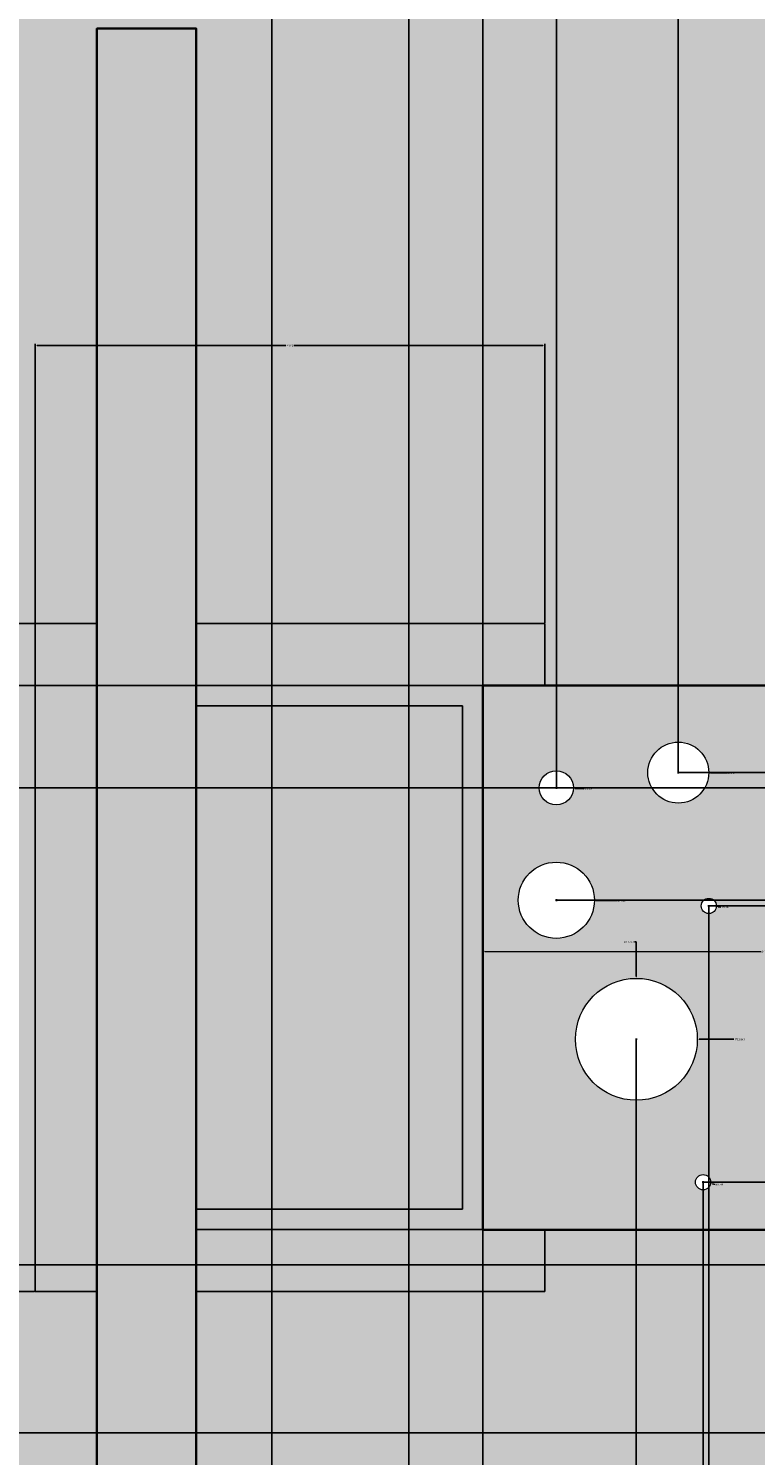
# Model space of a CAD drawing. Units: inches. Extents: x 73 to 607, y 92 to 651.
# Tile 3 of 18: x 298 to 368, y 173 to 311. Entities that reach past the tile are written whole.
import ezdxf

# ---------------------------------------------------------------- set-up
doc = ezdxf.new("R2010")
doc.units = ezdxf.units.IN
doc.header["$MEASUREMENT"] = 0
for name, color, linetype, lineweight in [('A-ANNO-DIMS', 2, 'Continuous', 18), ('A-ELEV', 7, 'Continuous', 35), ('A-ELEV-PANL', 7, 'Continuous', 18), ('A-ELEV-PATT-BKGD', 252, 'Continuous', 13), ('A-ELEV-PATT-FRAM', 38, 'Continuous', 13), ('A-ELEV-PATT-SHAD', 8, 'Continuous', 13), ('A-ELEV-PATT-WALL', 254, 'Continuous', 13), ('A-ELEV-PATT-WOOD', 32, 'Continuous', 13), ('A-GLAZ', 4, 'Continuous', 25), ('A-GLAZ-PATT', 7, 'Continuous', 13)]:
    doc.layers.add(name, color=color, linetype=linetype, lineweight=lineweight)
doc.styles.get("Standard").update_dxf_attribs({"font": 'arial.ttf'})
doc.dimstyles.get("Standard").update_dxf_attribs({"dimtxt": 0.18, "dimasz": 0.18, "dimexe": 0.18, "dimexo": 0.0625, "dimgap": 0.09, "dimtad": 0, "dimtih": 1, "dimtoh": 1, "dimdec": 4, "dimzin": 0, "dimdsep": 46, "dimtxsty": 'Standard', "dimcen": 0.09, "dimadec": 0, "dimazin": 0, "dimtfac": 1, "dimtdec": 4, "dimtofl": 0, "dimtmove": 0, "dimatfit": 3, "dimfxl": 1, "dimtolj": 1, "dimtzin": 0, "dimarcsym": 0})

# ---------------------------------------------------------------- blocks, each defined once
blk = doc.blocks.new('*D33')
at = {"layer": 'A-ANNO-DIMS', "color": 0, "lineweight": -2, "transparency": 16777216}
for p, q in [((298.36, 253.47), (298.36, 280.59)), ((298.54, 280.41), (322.73, 280.41)), ((347.69, 280.41), (323.49, 280.41)), ((347.87, 253.47), (347.87, 280.59))]:
    blk.add_line(p, q, dxfattribs=at)
at = {"layer": 'A-ANNO-DIMS', "color": 0, "transparency": 16777216}
for points in [[(298.54, 280.44), (298.54, 280.38), (298.36, 280.41)], [(347.69, 280.44), (347.69, 280.38), (347.87, 280.41)]]:
    blk.add_solid(points, dxfattribs=at)
at = {"layer": 'Defpoints', "color": 0, "transparency": 16777216}
for p in [(347.87, 280.41), (298.36, 253.41), (347.87, 253.41)]:
    blk.add_point(p, dxfattribs=at)
at = {"layer": 'A-ANNO-DIMS', "color": 0, "transparency": 16777216, "insert": (323.11, 280.41), "char_height": 0.18, "attachment_point": 5}
blk.add_mtext('\\A1;49.51', dxfattribs=at)
blk = doc.blocks.new('*D34')
at = {"layer": 'A-ANNO-DIMS', "color": 0, "lineweight": -2, "transparency": 16777216}
for p, q in [((298.29, 253.41), (271.18, 253.41)), ((271.36, 253.23), (271.36, 221.16)), ((271.36, 188.73), (271.36, 220.79)), ((298.29, 188.55), (271.18, 188.55))]:
    blk.add_line(p, q, dxfattribs=at)
at = {"layer": 'A-ANNO-DIMS', "color": 0, "transparency": 16777216}
for points in [[(271.33, 253.23), (271.39, 253.23), (271.36, 253.41)], [(271.33, 188.73), (271.39, 188.73), (271.36, 188.55)]]:
    blk.add_solid(points, dxfattribs=at)
at = {"layer": 'Defpoints', "color": 0, "transparency": 16777216}
for p in [(271.36, 253.41), (298.36, 253.41), (298.36, 188.55)]:
    blk.add_point(p, dxfattribs=at)
at = {"layer": 'A-ANNO-DIMS', "color": 0, "transparency": 16777216, "insert": (271.36, 220.98), "char_height": 0.18, "attachment_point": 5}
blk.add_mtext('\\A1;64.86', dxfattribs=at)
blk = doc.blocks.new('*D35')
at = {"layer": 'A-ANNO-DIMS', "color": 0, "lineweight": -2, "transparency": 16777216}
for p, q in [((341.87, 194.61), (341.87, 221.73)), ((342.05, 221.55), (368.89, 221.54)), ((396.52, 221.54), (369.68, 221.54)), ((396.69, 194.6), (396.7, 221.72))]:
    blk.add_line(p, q, dxfattribs=at)
at = {"layer": 'A-ANNO-DIMS', "color": 0, "transparency": 16777216}
for points in [[(342.05, 221.58), (342.05, 221.52), (341.87, 221.55)], [(396.52, 221.57), (396.52, 221.51), (396.7, 221.54)]]:
    blk.add_solid(points, dxfattribs=at)
at = {"layer": 'Defpoints', "color": 0, "transparency": 16777216}
for p in [(396.7, 221.54), (341.87, 194.55), (396.69, 194.54)]:
    blk.add_point(p, dxfattribs=at)
at = {"layer": 'A-ANNO-DIMS', "color": 0, "transparency": 16777216, "insert": (369.28, 221.54), "char_height": 0.18, "attachment_point": 5}
blk.add_mtext('\\A1;54.82', dxfattribs=at)
blk = doc.blocks.new('*D66')
at = {"layer": 'A-ANNO-DIMS', "color": 0, "lineweight": -2, "transparency": 16777216}
for p, q in [((356.68, 213.03), (356.86, 213.03)), ((356.77, 212.94), (356.77, 213.12)), ((366.25, 213.03), (362.88, 213.03))]:
    blk.add_line(p, q, dxfattribs=at)
at = {"layer": 'A-ANNO-DIMS', "color": 0, "transparency": 16777216}
blk.add_solid([(362.88, 213.06), (362.88, 213), (362.7, 213.03)], dxfattribs=at)
at = {"layer": 'Defpoints', "color": 0, "transparency": 16777216}
for p in [(350.85, 213.03), (362.7, 213.03)]:
    blk.add_point(p, dxfattribs=at)
at = {"layer": 'A-ANNO-DIMS', "color": 0, "transparency": 16777216, "insert": (366.81, 213.03), "char_height": 0.18, "attachment_point": 5}
blk.add_mtext('\\A1;∅11.843', dxfattribs=at)
blk = doc.blocks.new('*D77')
at = {"layer": 'A-ANNO-DIMS', "color": 0, "lineweight": -2, "transparency": 16777216}
for p, q in [((321.37, 356.99), (321.37, 116.02)), ((334.67, 320.14), (334.67, 116.02)), ((321.55, 116.2), (327.63, 116.2)), ((334.49, 116.2), (328.4, 116.2))]:
    blk.add_line(p, q, dxfattribs=at)
at = {"layer": 'A-ANNO-DIMS', "color": 0, "transparency": 16777216}
for points in [[(321.55, 116.23), (321.55, 116.17), (321.37, 116.2)], [(334.49, 116.23), (334.49, 116.17), (334.67, 116.2)]]:
    blk.add_solid(points, dxfattribs=at)
at = {"layer": 'Defpoints', "color": 0, "transparency": 16777216}
for p in [(321.37, 357.06), (334.67, 320.2), (321.37, 116.2)]:
    blk.add_point(p, dxfattribs=at)
at = {"layer": 'A-ANNO-DIMS', "color": 0, "transparency": 16777216, "insert": (328.02, 116.2), "char_height": 0.18, "attachment_point": 5}
blk.add_mtext('\\A1;13.30', dxfattribs=at)
blk = doc.blocks.new('*D81')
at = {"layer": 'A-ANNO-DIMS', "color": 0, "lineweight": -2, "transparency": 16777216}
for p, q in [((341.87, 247.47), (341.87, 650.98)), ((342.05, 650.8), (345.04, 650.8)), ((348.82, 650.8), (345.83, 650.8)), ((349, 237.52), (349, 650.98))]:
    blk.add_line(p, q, dxfattribs=at)
at = {"layer": 'A-ANNO-DIMS', "color": 0, "transparency": 16777216}
for points in [[(342.05, 650.83), (342.05, 650.77), (341.87, 650.8)], [(348.82, 650.83), (348.82, 650.77), (349, 650.8)]]:
    blk.add_solid(points, dxfattribs=at)
at = {"layer": 'Defpoints', "color": 0, "transparency": 16777216}
for p in [(349, 650.8), (341.87, 247.41), (349, 237.45)]:
    blk.add_point(p, dxfattribs=at)
at = {"layer": 'A-ANNO-DIMS', "color": 0, "transparency": 16777216, "insert": (345.43, 650.8), "char_height": 0.18, "attachment_point": 5}
blk.add_mtext('\\A1;7.128', dxfattribs=at)
blk = doc.blocks.new('*D82')
at = {"layer": 'A-ANNO-DIMS', "color": 0, "lineweight": -2, "transparency": 16777216}
for p, q in [((349, 237.52), (349, 650.98)), ((349.18, 650.8), (354.47, 650.8)), ((360.67, 650.8), (355.38, 650.8)), ((360.85, 239), (360.85, 650.98))]:
    blk.add_line(p, q, dxfattribs=at)
at = {"layer": 'A-ANNO-DIMS', "color": 0, "transparency": 16777216}
for points in [[(349.18, 650.83), (349.18, 650.77), (349, 650.8)], [(360.67, 650.83), (360.67, 650.77), (360.85, 650.8)]]:
    blk.add_solid(points, dxfattribs=at)
at = {"layer": 'Defpoints', "color": 0, "transparency": 16777216}
for p in [(360.85, 650.8), (360.85, 238.93), (349, 237.45)]:
    blk.add_point(p, dxfattribs=at)
at = {"layer": 'A-ANNO-DIMS', "color": 0, "transparency": 16777216, "insert": (354.92, 650.8), "char_height": 0.18, "attachment_point": 5}
blk.add_mtext('\\A1;11.852', dxfattribs=at)
blk = doc.blocks.new('*D83')
at = {"layer": 'A-ANNO-DIMS', "color": 0, "lineweight": -2, "transparency": 16777216}
for p, q in [((360.85, 239), (360.85, 650.98)), ((361.03, 650.8), (366.6, 650.8)), ((373.08, 650.8), (367.51, 650.8)), ((373.26, 231.41), (373.26, 650.98))]:
    blk.add_line(p, q, dxfattribs=at)
at = {"layer": 'A-ANNO-DIMS', "color": 0, "transparency": 16777216}
for points in [[(361.03, 650.83), (361.03, 650.77), (360.85, 650.8)], [(373.08, 650.83), (373.08, 650.77), (373.26, 650.8)]]:
    blk.add_solid(points, dxfattribs=at)
at = {"layer": 'Defpoints', "color": 0, "transparency": 16777216}
for p in [(373.26, 650.8), (360.85, 238.93), (373.26, 231.35)]:
    blk.add_point(p, dxfattribs=at)
at = {"layer": 'A-ANNO-DIMS', "color": 0, "transparency": 16777216, "insert": (367.05, 650.8), "char_height": 0.18, "attachment_point": 5}
blk.add_mtext('\\A1;12.408', dxfattribs=at)
blk = doc.blocks.new('*D86')
at = {"layer": 'A-ANNO-DIMS', "color": 0, "lineweight": -2, "transparency": 16777216}
for p, q in [((356.77, 212.97), (356.77, 116.02)), ((341.87, 194.47), (341.87, 116.02)), ((342.05, 116.2), (348.87, 116.2)), ((356.59, 116.2), (349.78, 116.2))]:
    blk.add_line(p, q, dxfattribs=at)
at = {"layer": 'A-ANNO-DIMS', "color": 0, "transparency": 16777216}
for points in [[(342.05, 116.23), (342.05, 116.17), (341.87, 116.2)], [(356.59, 116.23), (356.59, 116.17), (356.77, 116.2)]]:
    blk.add_solid(points, dxfattribs=at)
at = {"layer": 'Defpoints', "color": 0, "transparency": 16777216}
for p in [(356.77, 213.03), (341.87, 194.54), (356.77, 116.2)]:
    blk.add_point(p, dxfattribs=at)
at = {"layer": 'A-ANNO-DIMS', "color": 0, "transparency": 16777216, "insert": (349.32, 116.2), "char_height": 0.18, "attachment_point": 5}
blk.add_mtext('\\A1;14.906', dxfattribs=at)
blk = doc.blocks.new('*D87')
at = {"layer": 'A-ANNO-DIMS', "color": 0, "lineweight": -2, "transparency": 16777216}
for p, q in [((356.77, 212.97), (356.77, 116.02)), ((363.26, 199.09), (363.26, 116.02)), ((356.95, 116.2), (359.62, 116.2)), ((363.08, 116.2), (360.41, 116.2))]:
    blk.add_line(p, q, dxfattribs=at)
at = {"layer": 'A-ANNO-DIMS', "color": 0, "transparency": 16777216}
for points in [[(356.95, 116.23), (356.95, 116.17), (356.77, 116.2)], [(363.08, 116.23), (363.08, 116.17), (363.26, 116.2)]]:
    blk.add_solid(points, dxfattribs=at)
at = {"layer": 'Defpoints', "color": 0, "transparency": 16777216}
for p in [(356.77, 213.03), (363.26, 199.15), (363.26, 116.2)]:
    blk.add_point(p, dxfattribs=at)
at = {"layer": 'A-ANNO-DIMS', "color": 0, "transparency": 16777216, "insert": (360.02, 116.2), "char_height": 0.18, "attachment_point": 5}
blk.add_mtext('\\A1;6.482', dxfattribs=at)
blk = doc.blocks.new('*D88')
at = {"layer": 'A-ANNO-DIMS', "color": 0, "lineweight": -2, "transparency": 16777216}
for p, q in [((376.96, 209.08), (376.96, 116.02)), ((363.26, 199.09), (363.26, 116.02)), ((363.44, 116.2), (369.65, 116.2)), ((376.78, 116.2), (370.56, 116.2))]:
    blk.add_line(p, q, dxfattribs=at)
at = {"layer": 'A-ANNO-DIMS', "color": 0, "transparency": 16777216}
for points in [[(363.44, 116.23), (363.44, 116.17), (363.26, 116.2)], [(376.78, 116.23), (376.78, 116.17), (376.96, 116.2)]]:
    blk.add_solid(points, dxfattribs=at)
at = {"layer": 'Defpoints', "color": 0, "transparency": 16777216}
for p in [(376.96, 209.14), (363.26, 199.15), (376.96, 116.2)]:
    blk.add_point(p, dxfattribs=at)
at = {"layer": 'A-ANNO-DIMS', "color": 0, "transparency": 16777216, "insert": (370.11, 116.2), "char_height": 0.18, "attachment_point": 5}
blk.add_mtext('\\A1;13.704', dxfattribs=at)
blk = doc.blocks.new('*D91')
at = {"layer": 'A-ANNO-DIMS', "color": 0, "lineweight": -2, "transparency": 16777216}
for p, q in [((363.81, 225.92), (363.81, 116.02)), ((356.77, 212.97), (356.77, 116.02)), ((356.95, 116.2), (359.9, 116.2)), ((363.63, 116.2), (360.69, 116.2))]:
    blk.add_line(p, q, dxfattribs=at)
at = {"layer": 'A-ANNO-DIMS', "color": 0, "transparency": 16777216}
for points in [[(356.95, 116.23), (356.95, 116.17), (356.77, 116.2)], [(363.63, 116.23), (363.63, 116.17), (363.81, 116.2)]]:
    blk.add_solid(points, dxfattribs=at)
at = {"layer": 'Defpoints', "color": 0, "transparency": 16777216}
for p in [(363.81, 225.98), (356.77, 213.03), (363.81, 116.2)]:
    blk.add_point(p, dxfattribs=at)
at = {"layer": 'A-ANNO-DIMS', "color": 0, "transparency": 16777216, "insert": (360.29, 116.2), "char_height": 0.18, "attachment_point": 5}
blk.add_mtext('\\A1;7.037', dxfattribs=at)
blk = doc.blocks.new('*D92')
at = {"layer": 'A-ANNO-DIMS', "color": 0, "lineweight": -2, "transparency": 16777216}
for p, q in [((341.81, 247.41), (72.92, 247.41)), ((73.1, 247.23), (73.1, 242.61)), ((73.1, 237.63), (73.1, 242.25)), ((348.93, 237.45), (72.92, 237.45))]:
    blk.add_line(p, q, dxfattribs=at)
at = {"layer": 'A-ANNO-DIMS', "color": 0, "transparency": 16777216}
for points in [[(73.07, 247.23), (73.13, 247.23), (73.1, 247.41)], [(73.07, 237.63), (73.13, 237.63), (73.1, 237.45)]]:
    blk.add_solid(points, dxfattribs=at)
at = {"layer": 'Defpoints', "color": 0, "transparency": 16777216}
for p in [(341.87, 247.41), (73.1, 237.45), (349, 237.45)]:
    blk.add_point(p, dxfattribs=at)
at = {"layer": 'A-ANNO-DIMS', "color": 0, "transparency": 16777216, "insert": (73.1, 242.43), "char_height": 0.18, "attachment_point": 5}
blk.add_mtext('\\A1;9.95', dxfattribs=at)
blk = doc.blocks.new('*D93')
at = {"layer": 'A-ANNO-DIMS', "color": 0, "lineweight": -2, "transparency": 16777216}
for p, q in [((349.06, 237.45), (607.28, 237.45)), ((607.1, 237.27), (607.1, 232.18)), ((607.1, 226.72), (607.1, 231.81)), ((349.06, 226.54), (607.28, 226.54))]:
    blk.add_line(p, q, dxfattribs=at)
at = {"layer": 'A-ANNO-DIMS', "color": 0, "transparency": 16777216}
for points in [[(607.07, 237.27), (607.13, 237.27), (607.1, 237.45)], [(607.07, 226.72), (607.13, 226.72), (607.1, 226.54)]]:
    blk.add_solid(points, dxfattribs=at)
at = {"layer": 'Defpoints', "color": 0, "transparency": 16777216}
for p in [(349, 237.45), (349, 226.54), (607.1, 226.54)]:
    blk.add_point(p, dxfattribs=at)
at = {"layer": 'A-ANNO-DIMS', "color": 0, "transparency": 16777216, "insert": (607.1, 232), "char_height": 0.18, "attachment_point": 5}
blk.add_mtext('\\A1;10.917', dxfattribs=at)
blk = doc.blocks.new('*D94')
at = {"layer": 'A-ANNO-DIMS', "color": 0, "lineweight": -2, "transparency": 16777216}
for p, q in [((377.02, 209.14), (607.28, 209.14)), ((607.1, 208.96), (607.1, 204.33)), ((607.1, 199.33), (607.1, 203.97)), ((363.32, 199.15), (607.28, 199.15))]:
    blk.add_line(p, q, dxfattribs=at)
at = {"layer": 'A-ANNO-DIMS', "color": 0, "transparency": 16777216}
for points in [[(607.07, 208.96), (607.13, 208.96), (607.1, 209.14)], [(607.07, 199.33), (607.13, 199.33), (607.1, 199.15)]]:
    blk.add_solid(points, dxfattribs=at)
at = {"layer": 'Defpoints', "color": 0, "transparency": 16777216}
for p in [(376.96, 209.14), (363.26, 199.15), (607.1, 199.15)]:
    blk.add_point(p, dxfattribs=at)
at = {"layer": 'A-ANNO-DIMS', "color": 0, "transparency": 16777216, "insert": (607.1, 204.15), "char_height": 0.18, "attachment_point": 5}
blk.add_mtext('\\A1;9.992', dxfattribs=at)
blk = doc.blocks.new('*D95')
at = {"layer": 'A-ANNO-DIMS', "color": 0, "lineweight": -2, "transparency": 16777216}
for p, q in [((363.87, 225.98), (607.28, 225.98)), ((607.1, 225.8), (607.1, 212.75)), ((607.1, 199.33), (607.1, 212.38)), ((363.32, 199.15), (607.28, 199.15))]:
    blk.add_line(p, q, dxfattribs=at)
at = {"layer": 'A-ANNO-DIMS', "color": 0, "transparency": 16777216}
for points in [[(607.07, 225.8), (607.13, 225.8), (607.1, 225.98)], [(607.07, 199.33), (607.13, 199.33), (607.1, 199.15)]]:
    blk.add_solid(points, dxfattribs=at)
at = {"layer": 'Defpoints', "color": 0, "transparency": 16777216}
for p in [(363.81, 225.98), (607.1, 225.98), (363.26, 199.15)]:
    blk.add_point(p, dxfattribs=at)
at = {"layer": 'A-ANNO-DIMS', "color": 0, "transparency": 16777216, "insert": (607.1, 212.57), "char_height": 0.18, "attachment_point": 5}
blk.add_mtext('\\A1;26.83', dxfattribs=at)
blk = doc.blocks.new('*D96')
at = {"layer": 'A-ANNO-DIMS', "color": 0, "lineweight": -2, "transparency": 16777216}
for p, q in [((360.91, 238.93), (607.28, 238.93)), ((607.1, 238.75), (607.1, 232.64)), ((607.1, 226.16), (607.1, 232.28)), ((363.87, 225.98), (607.28, 225.98))]:
    blk.add_line(p, q, dxfattribs=at)
at = {"layer": 'A-ANNO-DIMS', "color": 0, "transparency": 16777216}
for points in [[(607.07, 238.75), (607.13, 238.75), (607.1, 238.93)], [(607.07, 226.16), (607.13, 226.16), (607.1, 225.98)]]:
    blk.add_solid(points, dxfattribs=at)
at = {"layer": 'Defpoints', "color": 0, "transparency": 16777216}
for p in [(360.85, 238.93), (607.1, 238.93), (363.81, 225.98)]:
    blk.add_point(p, dxfattribs=at)
at = {"layer": 'A-ANNO-DIMS', "color": 0, "transparency": 16777216, "insert": (607.1, 232.46), "char_height": 0.18, "attachment_point": 5}
blk.add_mtext('\\A1;12.953', dxfattribs=at)
blk = doc.blocks.new('*D119')
at = {"layer": 'A-ANNO-DIMS', "color": 0, "lineweight": -2, "transparency": 16777216}
for p, q in [((469.82, 191.14), (72.92, 191.14)), ((73.1, 190.96), (73.1, 183.15)), ((73.1, 174.98), (73.1, 182.79)), ((454.64, 174.8), (72.92, 174.8))]:
    blk.add_line(p, q, dxfattribs=at)
at = {"layer": 'A-ANNO-DIMS', "color": 0, "transparency": 16777216}
for points in [[(73.07, 190.96), (73.13, 190.96), (73.1, 191.14)], [(73.07, 174.98), (73.13, 174.98), (73.1, 174.8)]]:
    blk.add_solid(points, dxfattribs=at)
at = {"layer": 'Defpoints', "color": 0, "transparency": 16777216}
for p in [(73.1, 191.14), (469.88, 191.14), (454.7, 174.8)]:
    blk.add_point(p, dxfattribs=at)
at = {"layer": 'A-ANNO-DIMS', "color": 0, "transparency": 16777216, "insert": (73.1, 182.97), "char_height": 0.18, "attachment_point": 5}
blk.add_mtext('\\A1;16.34', dxfattribs=at)
blk = doc.blocks.new('*D142')
at = {"layer": 'A-ANNO-DIMS', "color": 0, "lineweight": -2, "transparency": 16777216}
for p, q in [((348.91, 237.45), (349.09, 237.45)), ((349, 237.36), (349, 237.54)), ((351.66, 237.37), (350.84, 237.39))]:
    blk.add_line(p, q, dxfattribs=at)
at = {"layer": 'A-ANNO-DIMS', "color": 0, "transparency": 16777216}
blk.add_solid([(350.84, 237.42), (350.84, 237.36), (350.66, 237.4)], dxfattribs=at)
at = {"layer": 'Defpoints', "color": 0, "transparency": 16777216}
for p in [(347.33, 237.51), (350.66, 237.4)]:
    blk.add_point(p, dxfattribs=at)
at = {"layer": 'A-ANNO-DIMS', "color": 0, "transparency": 16777216, "insert": (352.08, 237.37), "char_height": 0.18, "attachment_point": 5}
blk.add_mtext('\\A1;∅3.33', dxfattribs=at)
blk = doc.blocks.new('*D143')
at = {"layer": 'A-ANNO-DIMS', "color": 0, "lineweight": -2, "transparency": 16777216}
for p, q in [((360.76, 238.93), (360.94, 238.93)), ((360.85, 238.84), (360.85, 239.02)), ((365.59, 238.88), (363.99, 238.9))]:
    blk.add_line(p, q, dxfattribs=at)
at = {"layer": 'A-ANNO-DIMS', "color": 0, "transparency": 16777216}
blk.add_solid([(363.99, 238.93), (363.99, 238.87), (363.81, 238.9)], dxfattribs=at)
at = {"layer": 'Defpoints', "color": 0, "transparency": 16777216}
for p in [(357.89, 238.97), (363.81, 238.9)]:
    blk.add_point(p, dxfattribs=at)
at = {"layer": 'A-ANNO-DIMS', "color": 0, "transparency": 16777216, "insert": (366.06, 238.88), "char_height": 0.18, "attachment_point": 5}
blk.add_mtext('\\A1;∅5.921', dxfattribs=at)
blk = doc.blocks.new('*D147')
at = {"layer": 'A-ANNO-DIMS', "color": 0, "lineweight": -2, "transparency": 16777216}
for p, q in [((348.91, 226.54), (349.09, 226.54)), ((349, 226.45), (349, 226.63)), ((354.92, 226.48), (352.88, 226.5))]:
    blk.add_line(p, q, dxfattribs=at)
at = {"layer": 'A-ANNO-DIMS', "color": 0, "transparency": 16777216}
blk.add_solid([(352.88, 226.53), (352.88, 226.47), (352.7, 226.5)], dxfattribs=at)
at = {"layer": 'Defpoints', "color": 0, "transparency": 16777216}
for p in [(345.3, 226.57), (352.7, 226.5)]:
    blk.add_point(p, dxfattribs=at)
at = {"layer": 'A-ANNO-DIMS', "color": 0, "transparency": 16777216, "insert": (355.41, 226.48), "char_height": 0.18, "attachment_point": 5}
blk.add_mtext('\\A1;∅7.402', dxfattribs=at)
blk = doc.blocks.new('*D148')
at = {"layer": 'A-ANNO-DIMS', "color": 0, "lineweight": -2, "transparency": 16777216}
for p, q in [((363.72, 225.98), (363.9, 225.98)), ((363.81, 225.89), (363.81, 226.07)), ((364.99, 225.86), (364.73, 225.89))]:
    blk.add_line(p, q, dxfattribs=at)
at = {"layer": 'A-ANNO-DIMS', "color": 0, "transparency": 16777216}
blk.add_solid([(364.73, 225.92), (364.72, 225.86), (364.55, 225.91)], dxfattribs=at)
at = {"layer": 'Defpoints', "color": 0, "transparency": 16777216}
for p in [(363.08, 226.06), (364.55, 225.91)]:
    blk.add_point(p, dxfattribs=at)
at = {"layer": 'A-ANNO-DIMS', "color": 0, "transparency": 16777216, "insert": (365.41, 225.86), "char_height": 0.18, "attachment_point": 5}
blk.add_mtext('\\A1;∅1.48', dxfattribs=at)
blk = doc.blocks.new('*D150')
at = {"layer": 'A-ANNO-DIMS', "color": 0, "lineweight": -2, "transparency": 16777216}
for p, q in [((356.59, 222.5), (356.77, 222.5)), ((356.77, 222.5), (356.77, 219.13)), ((356.68, 213.03), (356.86, 213.03)), ((356.77, 212.94), (356.77, 213.12))]:
    blk.add_line(p, q, dxfattribs=at)
at = {"layer": 'A-ANNO-DIMS', "color": 0, "transparency": 16777216}
blk.add_solid([(356.8, 219.13), (356.74, 219.13), (356.77, 218.95)], dxfattribs=at)
at = {"layer": 'Defpoints', "color": 0, "transparency": 16777216}
for p in [(356.77, 218.95), (356.78, 207.11)]:
    blk.add_point(p, dxfattribs=at)
at = {"layer": 'A-ANNO-DIMS', "color": 0, "transparency": 16777216, "insert": (356.03, 222.5), "char_height": 0.18, "attachment_point": 5}
blk.add_mtext('\\A1;∅11.843', dxfattribs=at)
blk = doc.blocks.new('*D152')
at = {"layer": 'A-ANNO-DIMS', "color": 0, "lineweight": -2, "transparency": 16777216}
for p, q in [((363.17, 199.15), (363.35, 199.15)), ((363.26, 199.06), (363.26, 199.24)), ((364.42, 198.93), (364.16, 198.98))]:
    blk.add_line(p, q, dxfattribs=at)
at = {"layer": 'A-ANNO-DIMS', "color": 0, "transparency": 16777216}
blk.add_solid([(364.17, 199.01), (364.16, 198.95), (363.98, 199.01)], dxfattribs=at)
at = {"layer": 'Defpoints', "color": 0, "transparency": 16777216}
for p in [(362.53, 199.29), (363.98, 199.01)]:
    blk.add_point(p, dxfattribs=at)
at = {"layer": 'A-ANNO-DIMS', "color": 0, "transparency": 16777216, "insert": (364.84, 198.93), "char_height": 0.18, "attachment_point": 5}
blk.add_mtext('\\A1;∅1.48', dxfattribs=at)

msp = doc.modelspace()

# ---------------------------------------------------------------- hatches: boundary and pattern name
at = {"layer": 'A-ELEV-PATT-BKGD'}
h = msp.add_hatch(color=256, dxfattribs=at)
h.dxf.hatch_style = 1
h.paths.add_polyline_path([(321.3008, 479.2042), (312.3008, 479.2042), (312.3008, 478.7576), (312.3008, 412.636), (321.3008, 412.636)])
h.paths.add_polyline_path([(312.3008, 504.7576), (256.4726, 504.7576), (256.4726, 503.4576), (312.3008, 503.4576)], flags=17)
h.paths.add_polyline_path([(321.3008, 543.1576), (321.3008, 552.1576), (320.3257, 552.1576), (312.3008, 552.1576), (256.4726, 552.1576), (256.4726, 543.1576), (312.3008, 543.1576), (312.3008, 479.2042), (321.3008, 479.2042)])
h.paths.add_polyline_path([(451.5214, 412.636), (256.4726, 412.636), (256.4726, 403.636), (442.5214, 403.636), (442.5214, 320.2042), (206.1343, 320.2042), (206.1343, 320.9135), (206.1343, 403.636), (256.4726, 403.636), (256.4726, 412.636), (201.6343, 412.636), (201.6343, 320.9135), (201.6343, 320.2042), (201.6343, 311.2042), (256.4726, 311.2042), (451.5214, 311.2042)])
h.paths.add_polyline_path([(431.07, 258.6914), (369.5339, 258.6914), (369.5339, 247.4054), (396.692, 247.4054), (425.07, 247.4054), (425.07, 194.7312), (396.692, 194.6197), (396.692, 194.5366), (369.5339, 194.5366), (369.5339, 185.6619), (431.07, 185.6619)])
h.paths.add_polyline_path([(580.0983, 262.3024), (451.5214, 262.3024), (451.5214, 143.2042), (580.0983, 143.2042)])
h.paths.add_polyline_path([(454.7049, 174.802), (454.7049, 256.6321), (577.9249, 256.6321), (577.9249, 174.802)], flags=16)
h.paths.add_polyline_path([(465.9716, 191.1416, -1), (473.7874, 191.1416, -1)], flags=0)
h.paths.add_polyline_path([(490.5373, 181.6586, -1), (494.9999, 181.6586, -1)], flags=0)
h.paths.add_polyline_path([(476.2996, 209.8287, -1), (500.5844, 209.8287, -1)], flags=0)
h.paths.add_polyline_path([(505.3326, 194.7675, -1), (512.5843, 194.7675, -1)], flags=0)
h.paths.add_polyline_path([(520.9613, 186.679, -1), (526.544, 186.679, -1)], flags=0)
h.paths.add_polyline_path([(466.8103, 225.7267, -1), (470.1573, 225.7267, -1)], flags=0)
h.paths.add_polyline_path([(527.1059, 203.6926, -1), (536.0311, 203.6926, -1)], flags=0)
h.paths.add_polyline_path([(504.775, 232.6995, -1), (513.7002, 232.6995, -1)], flags=0)
h.paths.add_polyline_path([(546.9241, 183.611, -1), (554.7336, 183.611, -1)], flags=0)
h.paths.add_polyline_path([(459.5544, 243.856, -1), (466.8061, 243.856, -1)], flags=0)
h.paths.add_polyline_path([(476.3045, 246.924, -1), (488.5767, 246.924, -1)], flags=0)
h.paths.add_polyline_path([(529.9044, 226.8424, -1), (556.68, 226.8424, -1)], flags=0)
h.paths.add_polyline_path([(554.1814, 203.9716, -1), (561.4331, 203.9716, -1)], flags=0)
h.paths.add_polyline_path([(567.8561, 193.3729, -1), (570.6475, 193.3729, -1)], flags=0)
h.paths.add_polyline_path([(522.3584, 250.271, -1), (525.7053, 250.271, -1)], flags=0)
h.paths.add_polyline_path([(561.9965, 245.2506, -1), (567.5748, 245.2506, -1)], flags=0)
h.paths.add_polyline_path([(347.8686, 194.5366), (341.8686, 194.5366), (341.8686, 194.5452), (314.0144, 194.5452), (314.0144, 188.5452), (347.8686, 188.5452)])
h.paths.add_polyline_path([(347.8686, 253.4054), (314.0144, 253.4054), (314.0144, 247.4054), (341.8686, 247.4054), (347.8686, 247.4054)])
h.paths.add_polyline_path([(304.3559, 253.4054), (298.3559, 253.4054), (298.3559, 188.5452), (304.3559, 188.5452)])
h.paths.add_polyline_path([(450.6603, 552.1576), (369.9727, 552.1576), (369.9727, 479.2042), (374.4727, 479.2042), (374.4727, 547.6576), (446.1603, 547.6576), (446.1603, 479.2042), (450.6603, 479.2042)])
h.paths.add_polyline_path([(374.4727, 479.2042), (369.9727, 479.2042), (369.9727, 465.0632), (374.4727, 465.0632)])
h.paths.add_polyline_path([(450.6603, 479.2042), (446.1603, 479.2042), (446.1603, 465.0632), (450.6603, 465.0632)])
h.paths.add_polyline_path([(256.4726, 281.6039), (109.0983, 281.6039), (100.0983, 281.6039), (100.0983, 167.2042), (100.0983, 143.2042), (109.0983, 143.2042), (109.0983, 167.2042), (109.0983, 272.6039), (256.4726, 272.6039)])
at = {"layer": 'A-ELEV-PATT-FRAM'}
h = msp.add_hatch(color=256, dxfattribs=at)
h.dxf.hatch_style = 1
h.paths.add_polyline_path([(433.025, 403.636), (409.515, 403.636), (409.515, 342.1009), (411.515, 342.1009), (411.515, 401.636), (431.025, 401.636), (431.025, 342.1009), (433.025, 342.1009)])
h.paths.add_polyline_path([(433.025, 341.1009), (431.025, 341.1009), (431.025, 340.0025), (411.515, 340.0025), (411.515, 341.1009), (409.515, 341.1009), (409.515, 338.0025), (433.025, 338.0025)])
h.paths.add_polyline_path([(425.07, 247.4054), (396.692, 247.4054), (396.692, 194.6197), (425.07, 194.7312)])
h.paths.add_polyline_path([(423.07, 245.4054), (423.07, 196.7234), (398.8836, 196.6284), (398.692, 245.4054)], flags=16)
h.paths.add_polyline_path([(341.8686, 247.4054), (314.0144, 247.4054), (314.0144, 245.4054), (339.8686, 245.4054), (339.8686, 196.5452), (314.0144, 196.5452), (314.0144, 194.5452), (341.8686, 194.5452)])
h.paths.add_polyline_path([(372.3213, 383.1812), (350.3213, 383.1812), (350.3213, 342.1009), (372.3213, 342.1009)], flags=16)
h.paths.add_polyline_path([(376.3213, 389.1812), (346.3213, 389.1812), (346.3213, 342.1009), (350.3213, 342.1009), (350.3213, 383.1812), (372.3213, 383.1812), (372.3213, 342.1009), (376.3213, 342.1009)], flags=17)
h.paths.add_polyline_path([(375.3213, 362.2042, -1), (373.3213, 362.2042, -1)], flags=16)
h.paths.add_polyline_path([(379.3213, 392.2042), (343.3213, 392.2042), (343.3213, 342.1009), (346.3213, 342.1009), (346.3213, 389.1812), (376.3213, 389.1812), (376.3213, 342.1009), (379.3213, 342.1009)])
h.paths.add_polyline_path([(350.3213, 341.1009), (346.3213, 341.1009), (346.3213, 338.0025), (350.3213, 338.0025)])
h.paths.add_polyline_path([(346.3213, 341.1009), (343.3213, 341.1009), (343.3213, 338.0025), (346.3213, 338.0025)])
h.paths.add_polyline_path([(346.3213, 337.0025), (343.3213, 337.0025), (343.3213, 332.9397), (346.3213, 332.9397)])
h.paths.add_polyline_path([(350.3213, 337.0025), (346.3213, 337.0025), (346.3213, 332.9397), (350.3213, 332.9397)])
h.paths.add_polyline_path([(350.3213, 331.9397), (346.3213, 331.9397), (346.3213, 320.2042), (376.3213, 320.2042), (376.3213, 331.9397), (372.3213, 331.9397), (372.3213, 326.2042), (350.3213, 326.2042)])
h.paths.add_polyline_path([(372.3213, 337.0025), (350.3213, 337.0025), (350.3213, 332.9397), (372.3213, 332.9397)])
h.paths.add_polyline_path([(372.3213, 341.1009), (350.3213, 341.1009), (350.3213, 338.0025), (372.3213, 338.0025)])
h.paths.add_polyline_path([(376.3213, 341.1009), (372.3213, 341.1009), (372.3213, 338.0025), (376.3213, 338.0025)])
h.paths.add_polyline_path([(376.3213, 337.0025), (372.3213, 337.0025), (372.3213, 332.9397), (376.3213, 332.9397)])
h.paths.add_polyline_path([(379.3213, 341.1009), (376.3213, 341.1009), (376.3213, 338.0025), (379.3213, 338.0025)])
h.paths.add_polyline_path([(379.3213, 337.0025), (376.3213, 337.0025), (376.3213, 332.9397), (379.3213, 332.9397)])
h.paths.add_polyline_path([(379.3213, 331.9397), (376.3213, 331.9397), (376.3213, 320.2042), (379.3213, 320.2042)])
h.paths.add_polyline_path([(372.3213, 331.9397), (350.3213, 331.9397), (350.3213, 326.2042), (372.3213, 326.2042)], flags=17)
h.paths.add_polyline_path([(346.3213, 331.9397), (343.3213, 331.9397), (343.3213, 320.2042), (346.3213, 320.2042)])
at = {"layer": 'A-ELEV-PATT-SHAD'}
h = msp.add_hatch(color=256, dxfattribs=at)
h.dxf.hatch_style = 1
h.paths.add_polyline_path([(451.5214, 412.636), (256.4726, 412.636), (256.4726, 403.636), (442.5214, 403.636), (442.5214, 320.2042), (206.1343, 320.2042), (206.1343, 320.9135), (206.1343, 403.636), (256.4726, 403.636), (256.4726, 412.636), (201.6343, 412.636), (201.6343, 320.9135), (201.6343, 320.2042), (201.6343, 311.2042), (256.4726, 311.2042), (451.5214, 311.2042)])
h.paths.add_polyline_path([(580.0983, 262.3024), (451.5214, 262.3024), (451.5214, 143.2042), (580.0983, 143.2042)])
h.paths.add_polyline_path([(454.7049, 174.802), (454.7049, 256.6321), (577.9249, 256.6321), (577.9249, 174.802)], flags=16)
h.paths.add_polyline_path([(465.9716, 191.1416, -1), (473.7874, 191.1416, -1)], flags=0)
h.paths.add_polyline_path([(490.5373, 181.6586, -1), (494.9999, 181.6586, -1)], flags=0)
h.paths.add_polyline_path([(476.2996, 209.8287, -1), (500.5844, 209.8287, -1)], flags=0)
h.paths.add_polyline_path([(505.3326, 194.7675, -1), (512.5843, 194.7675, -1)], flags=0)
h.paths.add_polyline_path([(520.9613, 186.679, -1), (526.544, 186.679, -1)], flags=0)
h.paths.add_polyline_path([(466.8103, 225.7267, -1), (470.1573, 225.7267, -1)], flags=0)
h.paths.add_polyline_path([(527.1059, 203.6926, -1), (536.0311, 203.6926, -1)], flags=0)
h.paths.add_polyline_path([(459.5544, 243.856, -1), (466.8061, 243.856, -1)], flags=0)
h.paths.add_polyline_path([(504.775, 232.6995, -1), (513.7002, 232.6995, -1)], flags=0)
h.paths.add_polyline_path([(476.3045, 246.924, -1), (488.5767, 246.924, -1)], flags=0)
h.paths.add_polyline_path([(546.9241, 183.611, -1), (554.7336, 183.611, -1)], flags=0)
h.paths.add_polyline_path([(529.9044, 226.8424, -1), (556.68, 226.8424, -1)], flags=0)
h.paths.add_polyline_path([(554.1814, 203.9716, -1), (561.4331, 203.9716, -1)], flags=0)
h.paths.add_polyline_path([(522.3584, 250.271, -1), (525.7053, 250.271, -1)], flags=0)
h.paths.add_polyline_path([(567.8561, 193.3729, -1), (570.6475, 193.3729, -1)], flags=0)
h.paths.add_polyline_path([(561.9965, 245.2506, -1), (567.5748, 245.2506, -1)], flags=0)
h.paths.add_polyline_path([(431.07, 258.6914), (369.5339, 258.6914), (369.5339, 247.4054), (396.692, 247.4054), (425.07, 247.4054), (425.07, 194.7312), (396.692, 194.6197), (396.692, 194.5366), (369.5339, 194.5366), (369.5339, 185.6619), (431.07, 185.6619)])
h.paths.add_polyline_path([(347.8686, 253.4054), (314.0144, 253.4054), (314.0144, 247.4054), (341.8686, 247.4054), (347.8686, 247.4054)])
h.paths.add_polyline_path([(304.3559, 253.4054), (298.3559, 253.4054), (298.3559, 188.5452), (304.3559, 188.5452)])
h.paths.add_polyline_path([(347.8686, 194.5366), (341.8686, 194.5366), (341.8686, 194.5452), (314.0144, 194.5452), (314.0144, 188.5452), (347.8686, 188.5452)])
at = {"layer": 'A-ELEV-PATT-WALL'}
h = msp.add_hatch(color=256, dxfattribs=at)
h.dxf.hatch_style = 1
h.paths.add_polyline_path([(509.9692, 483.857), (450.6603, 483.857), (450.6603, 465.0632), (446.1603, 465.0632), (446.1603, 484.2142), (374.4727, 484.2142), (374.4727, 465.0632), (369.9727, 465.0632), (369.9727, 484.2142), (321.3008, 484.2142), (321.3008, 412.636), (451.5214, 412.636), (451.5214, 311.2042), (314.0144, 311.2042), (314.0144, 253.4054), (347.8686, 253.4054), (347.8686, 247.4054), (369.5339, 247.4054), (369.5339, 258.6914), (431.07, 258.6914), (431.07, 185.6619), (369.5339, 185.6619), (369.5339, 194.5366), (347.8686, 194.5366), (347.8686, 188.5452), (314.0144, 188.5452), (314.0144, 143.2042), (451.5214, 143.2042), (451.5214, 262.3024), (580.0983, 262.3024), (580.0983, 311.2042), (509.9692, 311.2042)])
h.paths.add_polyline_path([(304.3559, 311.2042), (256.4726, 311.2042), (256.4726, 167.2042), (256.4726, 143.2042), (304.3559, 143.2042), (304.3559, 188.5452), (298.3559, 188.5452), (298.3559, 253.4054), (304.3559, 253.4054)])
at = {"layer": 'A-ELEV-PATT-WOOD'}
h = msp.add_hatch(color=256, dxfattribs=at)
h.dxf.hatch_style = 1
h.paths.add_polyline_path([(314.0144, 311.2042), (304.3559, 311.2042), (304.3559, 143.2042), (314.0144, 143.2042)])
h = msp.add_hatch(color=256, dxfattribs=at)
h.dxf.hatch_style = 1
h.paths.add_polyline_path([(396.692, 247.4054), (341.8686, 247.4054), (341.8686, 194.5366), (375.5339, 194.5366), (396.692, 194.6197)])
h.paths.add_polyline_path([(390.6634, 232.4585, -1), (388.443, 232.4585, -1)], flags=16)
h.paths.add_polyline_path([(384.3667, 222.0962, -1), (381.4061, 222.0962, -1)], flags=16)
h.paths.add_polyline_path([(380.8505, 240.9703, -1), (383.8112, 240.9703, -1)], flags=16)
h.paths.add_polyline_path([(371.9613, 231.3482, -1), (374.5519, 231.3482, -1)], flags=16)
h.paths.add_polyline_path([(363.0718, 225.982, -1), (364.5521, 225.982, -1)], flags=16)
h.paths.add_polyline_path([(379.1808, 209.1433, -1), (374.7399, 209.1433, -1)], flags=16)
h.paths.add_polyline_path([(357.8883, 238.9349, -1), (363.8096, 238.9349, -1)], flags=16)
h.paths.add_polyline_path([(362.6961, 213.0292, -1), (350.8535, 213.0292, -1)], flags=16)
h.paths.add_polyline_path([(388.8114, 200.0764, -1), (386.2208, 200.0764, -1)], flags=16)
h.paths.add_polyline_path([(352.6976, 226.5372, -1), (345.296, 226.5372, -1)], flags=16)
h.paths.add_polyline_path([(347.3301, 237.4546, -1), (350.6635, 237.4546, -1)], flags=16)
h.paths.add_polyline_path([(363.9971, 199.1512, -1), (362.5156, 199.1512, -1)], flags=16)
at = {"layer": 'A-GLAZ-PATT'}
h = msp.add_hatch(color=256, dxfattribs=at)
h.dxf.hatch_style = 1
h.set_gradient(color1=(0, 0, 255))
h.paths.add_polyline_path([(339.8686, 245.4054), (314.0144, 245.4054), (314.0144, 196.5452), (339.8686, 196.5452)])

# ---------------------------------------------------------------- linework, layer by layer
at = {"layer": 'A-ELEV'}
for points in [[(304.3559, 143.2042), (314.0144, 143.2042), (314.0144, 311.2042), (304.3559, 311.2042)], [(341.8686, 247.4054), (396.692, 247.4054), (396.692, 194.5366), (341.8686, 194.5366)]]:
    msp.add_lwpolyline(points, close=True, dxfattribs=at)
at = {"layer": 'A-ELEV-PANL'}
for centre, radius in [((360.8489, 238.9349), 2.9606), ((348.9968, 237.4546), 1.6667), ((348.9968, 226.5372), 3.7008), ((363.8119, 225.982), 0.7402), ((356.7748, 213.0292), 5.9213), ((363.2564, 199.1512), 0.7408)]:
    msp.add_circle(centre, radius, dxfattribs=at)
at = {"layer": 'A-GLAZ'}
for points in [[(304.3559, 188.5452), (298.3559, 188.5452), (298.3559, 253.4054), (304.3559, 253.4054)], [(314.0144, 253.4054), (347.8686, 253.4054), (347.8686, 247.4054)], [(304.3559, 194.5452), (304.3559, 247.4054)], [(314.0144, 247.4054), (341.8686, 247.4054), (341.8686, 194.5452), (314.0144, 194.5452)], [(314.0144, 245.4054), (339.8686, 245.4054), (339.8686, 196.5452), (314.0144, 196.5452)], [(347.8686, 194.5366), (347.8686, 188.5452), (314.0144, 188.5452)]]:
    msp.add_lwpolyline(points, dxfattribs=at)

# ---------------------------------------------------------------- dimensions: what is measured, and where the dimension line sits
at = {"layer": 'A-ANNO-DIMS'}
for base, p1, p2, override, picture, middle in [((348.9968, 650.801), (341.8686, 247.4054), (348.9968, 237.4546), {"dimdec": 3, "dimlfac": 1, "dimrnd": 0, "dimzin": 0, "dimdsep": 46, "dimlunit": 2}, '*D81', (345.4327, 650.801)), ((360.8489, 650.801), (348.9968, 237.4546), (360.8489, 238.9349), {"dimdec": 3, "dimlfac": 1, "dimrnd": 0, "dimzin": 0, "dimdsep": 46, "dimlunit": 2}, '*D82', (354.9229, 650.801)), ((373.2566, 650.801), (360.8489, 238.9349), (373.2566, 231.3482), {"dimdec": 3, "dimlfac": 1, "dimrnd": 0, "dimzin": 0, "dimdsep": 46, "dimlunit": 2}, '*D83', (367.0527, 650.801)), ((321.3681, 116.2042), (334.6695, 320.2042), (321.3681, 357.0571), {"dimdec": 2, "dimlfac": 1, "dimrnd": 0, "dimzin": 0, "dimdsep": 46, "dimlunit": 2}, '*D77', (328.0188, 116.2042)), ((347.8686, 280.4054), (298.3559, 253.4054), (347.8686, 253.4054), {"dimdec": 2, "dimlfac": 1, "dimrnd": 0, "dimzin": 0, "dimdsep": 46, "dimlunit": 2}, '*D33', (323.1122, 280.4054)), ((363.8119, 116.2042), (356.7748, 213.0292), (363.8119, 225.982), {"dimdec": 3, "dimlfac": 1, "dimrnd": 0, "dimzin": 0, "dimdsep": 46, "dimlunit": 2}, '*D91', (360.2933, 116.2042)), ((356.7748, 116.2042), (341.8686, 194.5366), (356.7748, 213.0292), {"dimdec": 3, "dimlfac": 1, "dimrnd": 0, "dimzin": 0, "dimdsep": 46, "dimlunit": 2}, '*D86', (349.3217, 116.2042)), ((363.2564, 116.2042), (356.7748, 213.0292), (363.2564, 199.1512), {"dimdec": 3, "dimlfac": 1, "dimrnd": 0, "dimzin": 0, "dimdsep": 46, "dimlunit": 2}, '*D87', (360.0156, 116.2042)), ((376.9603, 116.2042), (363.2564, 199.1512), (376.9603, 209.1433), {"dimdec": 3, "dimlfac": 1, "dimrnd": 0, "dimzin": 0, "dimdsep": 46, "dimlunit": 2}, '*D88', (370.1084, 116.2042))]:
    dim = msp.add_linear_dim(base=base, p1=p1, p2=p2, dimstyle='Standard', override=override, dxfattribs=at)
    dim.commit()
    dim.dimension.update_dxf_attribs({"geometry": picture, "text_midpoint": middle})
for base, p1, p2, angle, override, picture, middle in [((271.3559, 253.4054), (298.3559, 188.5452), (298.3559, 253.4054), 90, {"dimdec": 2, "dimlfac": 1, "dimrnd": 0, "dimzin": 0, "dimdsep": 46, "dimlunit": 2}, '*D34', (271.3559, 220.9753)), ((73.0983, 237.4546), (341.8686, 247.4054), (348.9968, 237.4546), 90, {"dimdec": 2, "dimlfac": 1, "dimrnd": 0, "dimzin": 0, "dimdsep": 46, "dimlunit": 2}, '*D92', (73.0983, 242.43)), ((607.0983, 238.9349), (363.8119, 225.982), (360.8489, 238.9349), 90, {"dimdec": 3, "dimlfac": 1, "dimrnd": 0, "dimzin": 0, "dimdsep": 46, "dimlunit": 2}, '*D96', (607.0983, 232.4585)), ((607.0983, 226.5372), (348.9968, 237.4546), (348.9968, 226.5372), 90, {"dimdec": 3, "dimlfac": 1, "dimrnd": 0, "dimzin": 0, "dimdsep": 46, "dimlunit": 2}, '*D93', (607.0983, 231.9959)), ((607.0983, 225.982), (363.2564, 199.1512), (363.8119, 225.982), 90, {"dimdec": 2, "dimlfac": 1, "dimrnd": 0, "dimzin": 0, "dimdsep": 46, "dimlunit": 2}, '*D95', (607.0983, 212.5666)), ((396.6962, 221.5366), (341.8686, 194.5452), (396.692, 194.5366), 359.991065, {"dimdec": 2, "dimlfac": 1, "dimrnd": 0, "dimzin": 0, "dimdsep": 46, "dimlunit": 2}, '*D35', (369.2845, 221.5409)), ((607.0983, 199.1512), (376.9603, 209.1433), (363.2564, 199.1512), 90, {"dimdec": 3, "dimlfac": 1, "dimrnd": 0, "dimzin": 0, "dimdsep": 46, "dimlunit": 2}, '*D94', (607.0983, 204.1472)), ((73.0983, 191.1416), (454.7049, 174.802), (469.8795, 191.1416), 90, {"dimdec": 2, "dimlfac": 1, "dimrnd": 0, "dimzin": 0, "dimdsep": 46, "dimlunit": 2}, '*D119', (73.0983, 182.9718))]:
    dim = msp.add_linear_dim(base=base, p1=p1, p2=p2, angle=angle, dimstyle='Standard', override=override, dxfattribs=at)
    dim.commit()
    dim.dimension.update_dxf_attribs({"geometry": picture, "text_midpoint": middle})
for p1, p2, override, picture, middle in [((357.8885, 238.969), (363.8094, 238.9008), {"dimdec": 3, "dimlfac": 1, "dimrnd": 0, "dimzin": 0, "dimdsep": 46, "dimlunit": 2}, '*D143', (365.5856, 238.8804)), ((347.331, 237.5089), (350.6626, 237.4002), {"dimdec": 2, "dimlfac": 1, "dimrnd": 0, "dimzin": 0, "dimdsep": 46, "dimlunit": 2}, '*D142', (351.6621, 237.3676)), ((345.2962, 226.5742), (352.6974, 226.5001), {"dimdec": 3, "dimlfac": 1, "dimrnd": 0, "dimzin": 0, "dimdsep": 46, "dimlunit": 2}, '*D147', (354.9178, 226.4779)), ((363.0755, 226.0559), (364.5484, 225.9082), {"dimdec": 2, "dimlfac": 1, "dimrnd": 0, "dimzin": 0, "dimdsep": 46, "dimlunit": 2}, '*D148', (364.9903, 225.8639)), ((356.7795, 207.1079), (356.77, 218.9505), {"dimdec": 3, "dimlfac": 1, "dimrnd": 0, "dimzin": 0, "dimdsep": 46, "dimlunit": 2}, '*D150', (356.0256, 222.5033)), ((350.8535, 213.0294), (362.6961, 213.029), {"dimdec": 3, "dimlfac": 1, "dimrnd": 0, "dimzin": 0, "dimdsep": 46, "dimlunit": 2}, '*D66', (366.2488, 213.0289)), ((362.5287, 199.2897), (363.984, 199.0126), {"dimdec": 2, "dimlfac": 1, "dimrnd": 0, "dimzin": 0, "dimdsep": 46, "dimlunit": 2}, '*D152', (364.4206, 198.9294))]:
    dim = msp.add_diameter_dim_2p(p1=p1, p2=p2, dimstyle='Standard', override=override, dxfattribs=at)
    dim.commit()
    dim.dimension.update_dxf_attribs({"geometry": picture, "text_midpoint": middle, "dimtype": 163})

doc.saveas('drawing.dxf')
